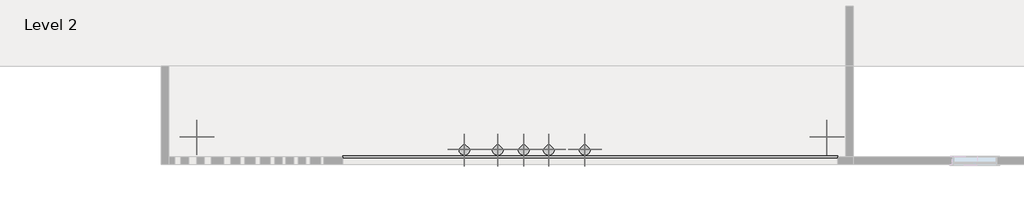
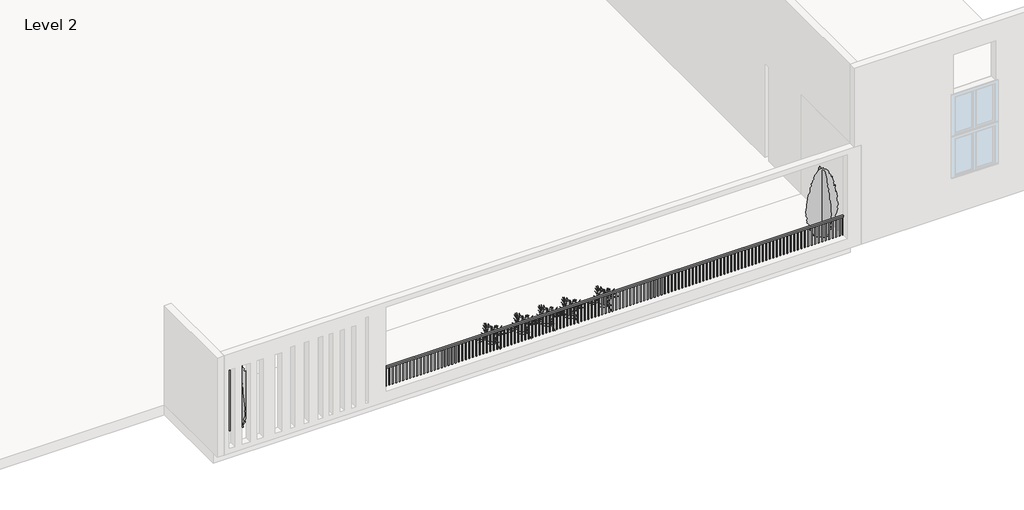
# One storey, part 2 of 2: 7 geographic elements, 1 railing.
"""IFC4 building model written with IfcOpenShell, lengths in millimetres."""

from ifc_helpers import new_model, si_unit, frame, origin, place, context, project, spatial, polyline, outline, extrude, transform, mapped, element, save
from components import rpc_plant_tropical_agave_1_5_93a2a214, rpc_tree_conifer_chinese_juniper_7_1b9786cd

model = new_model("IFC4")

# Units and contexts
model_context = context("Model", 3, world=origin())
ifc_project = project(units=[si_unit("LENGTHUNIT", "METRE", prefix="MILLI")], contexts=[model_context])

# Site, building, storey
site = spatial("IfcSite", under=ifc_project)
building = spatial("IfcBuilding", under=site)
storey = spatial("IfcBuildingStorey", under=building, Name="Level 2", Elevation=3200.4)

# Geographic elements
placement = place(None, origin())
rpc_plant_tropical_agave_1_5_shape = rpc_plant_tropical_agave_1_5_93a2a214(model_context)
element("IfcGeographicElement", 1, ObjectType="RPC Plant - Tropical : Agave - 1.5'", at=placement, inside=storey, context=model_context, shape_type="MappedRepresentation", body=[
    mapped(rpc_plant_tropical_agave_1_5_shape, transform((-1518.2073975, -18818.2462052, 3657.6), x_axis=(1.0, 0.0, 0.0), y_axis=(0.0, 1.0, 0.0), z_axis=(0.0, 0.0, 1.0))),
])
element("IfcGeographicElement", 2, ObjectType="RPC Plant - Tropical : Agave - 1.5'", at=placement, inside=storey, context=model_context, shape_type="MappedRepresentation", body=[
    mapped(rpc_plant_tropical_agave_1_5_shape, transform((-616.8826315, -18818.2462052, 3657.6), x_axis=(1.0, 0.0, 0.0), y_axis=(0.0, 1.0, 0.0), z_axis=(0.0, 0.0, 1.0))),
])
element("IfcGeographicElement", 3, ObjectType="RPC Plant - Tropical : Agave - 1.5'", at=placement, inside=storey, context=model_context, shape_type="MappedRepresentation", body=[
    mapped(rpc_plant_tropical_agave_1_5_shape, transform((88.759784, -18818.2462052, 3657.6), x_axis=(1.0, 0.0, 0.0), y_axis=(0.0, 1.0, 0.0), z_axis=(0.0, 0.0, 1.0))),
])
element("IfcGeographicElement", 4, ObjectType="RPC Plant - Tropical : Agave - 1.5'", at=placement, inside=storey, context=model_context, shape_type="MappedRepresentation", body=[
    mapped(rpc_plant_tropical_agave_1_5_shape, transform((764.7533585, -18818.2462052, 3657.6), x_axis=(1.0, 0.0, 0.0), y_axis=(0.0, 1.0, 0.0), z_axis=(0.0, 0.0, 1.0))),
])
element("IfcGeographicElement", 5, ObjectType="RPC Plant - Tropical : Agave - 1.5'", at=placement, inside=storey, context=model_context, shape_type="MappedRepresentation", body=[
    mapped(rpc_plant_tropical_agave_1_5_shape, transform((1745.1760973, -18818.2462052, 3657.6), x_axis=(1.0, 0.0, 0.0), y_axis=(0.0, 1.0, 0.0), z_axis=(0.0, 0.0, 1.0))),
])
rpc_tree_conifer_chinese_juniper_7_shape = rpc_tree_conifer_chinese_juniper_7_1b9786cd(model_context)
element("IfcGeographicElement", 6, ObjectType="RPC Tree - Conifer : Chinese Juniper - 7'", at=placement, inside=storey, context=model_context, shape_type="MappedRepresentation", body=[
    mapped(rpc_tree_conifer_chinese_juniper_7_shape, transform((8298.1794262, -18476.470124, 3200.4), x_axis=(1.0, 0.0, 0.0), y_axis=(0.0, 1.0, 0.0), z_axis=(0.0, 0.0, 1.0))),
])
element("IfcGeographicElement", 7, ObjectType="RPC Tree - Conifer : Chinese Juniper - 7'", at=placement, inside=storey, context=model_context, shape_type="MappedRepresentation", body=[
    mapped(rpc_tree_conifer_chinese_juniper_7_shape, transform((-8770.6205738, -18476.470124, 3200.4), x_axis=(1.0, 0.0, 0.0), y_axis=(0.0, 1.0, 0.0), z_axis=(0.0, 0.0, 1.0))),
])

# Railing
element("IfcRailing", 8, ObjectType="Handrail - Rectangular", at=placement, inside=storey, context=model_context, shape_type="SweptSolid", body=[
    extrude(outline(polyline([(-4809.1668389, -19046.8462052), (-4809.1668389, -18996.0462052), (8602.0331611, -18996.0462052), (8602.0331611, -19046.8462052), (-4809.1668389, -19046.8462052)])), frame((0.0, 0.0, 4064.0), z_axis=(0.0, 0.0, 1.0), x_axis=(1.0, 0.0, 0.0)), (0.0, 0.0, 1.0), 50.8),
    extrude(outline(polyline([(8490.9081611, -19030.9712052), (8490.9081611, -19011.9212052), (8509.9581611, -19011.9212052), (8509.9581611, -19030.9712052), (8490.9081611, -19030.9712052)])), frame((0.0, 0.0, 3200.4), z_axis=(0.0, 0.0, 1.0), x_axis=(1.0, 0.0, 0.0)), (0.0, 0.0, 1.0), 863.6),
    extrude(outline(polyline([(8389.3081611, -19030.9712052), (8389.3081611, -19011.9212052), (8408.3581611, -19011.9212052), (8408.3581611, -19030.9712052), (8389.3081611, -19030.9712052)])), frame((0.0, 0.0, 3200.4), z_axis=(0.0, 0.0, 1.0), x_axis=(1.0, 0.0, 0.0)), (0.0, 0.0, 1.0), 863.6),
    extrude(outline(polyline([(8287.7081611, -19030.9712052), (8287.7081611, -19011.9212052), (8306.7581611, -19011.9212052), (8306.7581611, -19030.9712052), (8287.7081611, -19030.9712052)])), frame((0.0, 0.0, 3200.4), z_axis=(0.0, 0.0, 1.0), x_axis=(1.0, 0.0, 0.0)), (0.0, 0.0, 1.0), 863.6),
    extrude(outline(polyline([(8186.1081611, -19030.9712052), (8186.1081611, -19011.9212052), (8205.1581611, -19011.9212052), (8205.1581611, -19030.9712052), (8186.1081611, -19030.9712052)])), frame((0.0, 0.0, 3200.4), z_axis=(0.0, 0.0, 1.0), x_axis=(1.0, 0.0, 0.0)), (0.0, 0.0, 1.0), 863.6),
    extrude(outline(polyline([(8084.5081611, -19030.9712052), (8084.5081611, -19011.9212052), (8103.5581611, -19011.9212052), (8103.5581611, -19030.9712052), (8084.5081611, -19030.9712052)])), frame((0.0, 0.0, 3200.4), z_axis=(0.0, 0.0, 1.0), x_axis=(1.0, 0.0, 0.0)), (0.0, 0.0, 1.0), 863.6),
    extrude(outline(polyline([(7982.9081611, -19030.9712052), (7982.9081611, -19011.9212052), (8001.9581611, -19011.9212052), (8001.9581611, -19030.9712052), (7982.9081611, -19030.9712052)])), frame((0.0, 0.0, 3200.4), z_axis=(0.0, 0.0, 1.0), x_axis=(1.0, 0.0, 0.0)), (0.0, 0.0, 1.0), 863.6),
    extrude(outline(polyline([(7881.3081611, -19030.9712052), (7881.3081611, -19011.9212052), (7900.3581611, -19011.9212052), (7900.3581611, -19030.9712052), (7881.3081611, -19030.9712052)])), frame((0.0, 0.0, 3200.4), z_axis=(0.0, 0.0, 1.0), x_axis=(1.0, 0.0, 0.0)), (0.0, 0.0, 1.0), 863.6),
    extrude(outline(polyline([(7779.7081611, -19030.9712052), (7779.7081611, -19011.9212052), (7798.7581611, -19011.9212052), (7798.7581611, -19030.9712052), (7779.7081611, -19030.9712052)])), frame((0.0, 0.0, 3200.4), z_axis=(0.0, 0.0, 1.0), x_axis=(1.0, 0.0, 0.0)), (0.0, 0.0, 1.0), 863.6),
    extrude(outline(polyline([(7678.1081611, -19030.9712052), (7678.1081611, -19011.9212052), (7697.1581611, -19011.9212052), (7697.1581611, -19030.9712052), (7678.1081611, -19030.9712052)])), frame((0.0, 0.0, 3200.4), z_axis=(0.0, 0.0, 1.0), x_axis=(1.0, 0.0, 0.0)), (0.0, 0.0, 1.0), 863.6),
    extrude(outline(polyline([(7576.5081611, -19030.9712052), (7576.5081611, -19011.9212052), (7595.5581611, -19011.9212052), (7595.5581611, -19030.9712052), (7576.5081611, -19030.9712052)])), frame((0.0, 0.0, 3200.4), z_axis=(0.0, 0.0, 1.0), x_axis=(1.0, 0.0, 0.0)), (0.0, 0.0, 1.0), 863.6),
    extrude(outline(polyline([(7474.9081611, -19030.9712052), (7474.9081611, -19011.9212052), (7493.9581611, -19011.9212052), (7493.9581611, -19030.9712052), (7474.9081611, -19030.9712052)])), frame((0.0, 0.0, 3200.4), z_axis=(0.0, 0.0, 1.0), x_axis=(1.0, 0.0, 0.0)), (0.0, 0.0, 1.0), 863.6),
    extrude(outline(polyline([(7373.3081611, -19030.9712052), (7373.3081611, -19011.9212052), (7392.3581611, -19011.9212052), (7392.3581611, -19030.9712052), (7373.3081611, -19030.9712052)])), frame((0.0, 0.0, 3200.4), z_axis=(0.0, 0.0, 1.0), x_axis=(1.0, 0.0, 0.0)), (0.0, 0.0, 1.0), 863.6),
    extrude(outline(polyline([(7271.7081611, -19030.9712052), (7271.7081611, -19011.9212052), (7290.7581611, -19011.9212052), (7290.7581611, -19030.9712052), (7271.7081611, -19030.9712052)])), frame((0.0, 0.0, 3200.4), z_axis=(0.0, 0.0, 1.0), x_axis=(1.0, 0.0, 0.0)), (0.0, 0.0, 1.0), 863.6),
    extrude(outline(polyline([(7170.1081611, -19030.9712052), (7170.1081611, -19011.9212052), (7189.1581611, -19011.9212052), (7189.1581611, -19030.9712052), (7170.1081611, -19030.9712052)])), frame((0.0, 0.0, 3200.4), z_axis=(0.0, 0.0, 1.0), x_axis=(1.0, 0.0, 0.0)), (0.0, 0.0, 1.0), 863.6),
    extrude(outline(polyline([(7068.5081611, -19030.9712052), (7068.5081611, -19011.9212052), (7087.5581611, -19011.9212052), (7087.5581611, -19030.9712052), (7068.5081611, -19030.9712052)])), frame((0.0, 0.0, 3200.4), z_axis=(0.0, 0.0, 1.0), x_axis=(1.0, 0.0, 0.0)), (0.0, 0.0, 1.0), 863.6),
    extrude(outline(polyline([(6966.9081611, -19030.9712052), (6966.9081611, -19011.9212052), (6985.9581611, -19011.9212052), (6985.9581611, -19030.9712052), (6966.9081611, -19030.9712052)])), frame((0.0, 0.0, 3200.4), z_axis=(0.0, 0.0, 1.0), x_axis=(1.0, 0.0, 0.0)), (0.0, 0.0, 1.0), 863.6),
    extrude(outline(polyline([(6865.3081611, -19030.9712052), (6865.3081611, -19011.9212052), (6884.3581611, -19011.9212052), (6884.3581611, -19030.9712052), (6865.3081611, -19030.9712052)])), frame((0.0, 0.0, 3200.4), z_axis=(0.0, 0.0, 1.0), x_axis=(1.0, 0.0, 0.0)), (0.0, 0.0, 1.0), 863.6),
    extrude(outline(polyline([(6763.7081611, -19030.9712052), (6763.7081611, -19011.9212052), (6782.7581611, -19011.9212052), (6782.7581611, -19030.9712052), (6763.7081611, -19030.9712052)])), frame((0.0, 0.0, 3200.4), z_axis=(0.0, 0.0, 1.0), x_axis=(1.0, 0.0, 0.0)), (0.0, 0.0, 1.0), 863.6),
    extrude(outline(polyline([(6662.1081611, -19030.9712052), (6662.1081611, -19011.9212052), (6681.1581611, -19011.9212052), (6681.1581611, -19030.9712052), (6662.1081611, -19030.9712052)])), frame((0.0, 0.0, 3200.4), z_axis=(0.0, 0.0, 1.0), x_axis=(1.0, 0.0, 0.0)), (0.0, 0.0, 1.0), 863.6),
    extrude(outline(polyline([(6560.5081611, -19030.9712052), (6560.5081611, -19011.9212052), (6579.5581611, -19011.9212052), (6579.5581611, -19030.9712052), (6560.5081611, -19030.9712052)])), frame((0.0, 0.0, 3200.4), z_axis=(0.0, 0.0, 1.0), x_axis=(1.0, 0.0, 0.0)), (0.0, 0.0, 1.0), 863.6),
    extrude(outline(polyline([(6458.9081611, -19030.9712052), (6458.9081611, -19011.9212052), (6477.9581611, -19011.9212052), (6477.9581611, -19030.9712052), (6458.9081611, -19030.9712052)])), frame((0.0, 0.0, 3200.4), z_axis=(0.0, 0.0, 1.0), x_axis=(1.0, 0.0, 0.0)), (0.0, 0.0, 1.0), 863.6),
    extrude(outline(polyline([(6357.3081611, -19030.9712052), (6357.3081611, -19011.9212052), (6376.3581611, -19011.9212052), (6376.3581611, -19030.9712052), (6357.3081611, -19030.9712052)])), frame((0.0, 0.0, 3200.4), z_axis=(0.0, 0.0, 1.0), x_axis=(1.0, 0.0, 0.0)), (0.0, 0.0, 1.0), 863.6),
    extrude(outline(polyline([(6255.7081611, -19030.9712052), (6255.7081611, -19011.9212052), (6274.7581611, -19011.9212052), (6274.7581611, -19030.9712052), (6255.7081611, -19030.9712052)])), frame((0.0, 0.0, 3200.4), z_axis=(0.0, 0.0, 1.0), x_axis=(1.0, 0.0, 0.0)), (0.0, 0.0, 1.0), 863.6),
    extrude(outline(polyline([(6154.1081611, -19030.9712052), (6154.1081611, -19011.9212052), (6173.1581611, -19011.9212052), (6173.1581611, -19030.9712052), (6154.1081611, -19030.9712052)])), frame((0.0, 0.0, 3200.4), z_axis=(0.0, 0.0, 1.0), x_axis=(1.0, 0.0, 0.0)), (0.0, 0.0, 1.0), 863.6),
    extrude(outline(polyline([(6052.5081611, -19030.9712052), (6052.5081611, -19011.9212052), (6071.5581611, -19011.9212052), (6071.5581611, -19030.9712052), (6052.5081611, -19030.9712052)])), frame((0.0, 0.0, 3200.4), z_axis=(0.0, 0.0, 1.0), x_axis=(1.0, 0.0, 0.0)), (0.0, 0.0, 1.0), 863.6),
    extrude(outline(polyline([(5950.9081611, -19030.9712052), (5950.9081611, -19011.9212052), (5969.9581611, -19011.9212052), (5969.9581611, -19030.9712052), (5950.9081611, -19030.9712052)])), frame((0.0, 0.0, 3200.4), z_axis=(0.0, 0.0, 1.0), x_axis=(1.0, 0.0, 0.0)), (0.0, 0.0, 1.0), 863.6),
    extrude(outline(polyline([(5849.3081611, -19030.9712052), (5849.3081611, -19011.9212052), (5868.3581611, -19011.9212052), (5868.3581611, -19030.9712052), (5849.3081611, -19030.9712052)])), frame((0.0, 0.0, 3200.4), z_axis=(0.0, 0.0, 1.0), x_axis=(1.0, 0.0, 0.0)), (0.0, 0.0, 1.0), 863.6),
    extrude(outline(polyline([(5747.7081611, -19030.9712052), (5747.7081611, -19011.9212052), (5766.7581611, -19011.9212052), (5766.7581611, -19030.9712052), (5747.7081611, -19030.9712052)])), frame((0.0, 0.0, 3200.4), z_axis=(0.0, 0.0, 1.0), x_axis=(1.0, 0.0, 0.0)), (0.0, 0.0, 1.0), 863.6),
    extrude(outline(polyline([(5646.1081611, -19030.9712052), (5646.1081611, -19011.9212052), (5665.1581611, -19011.9212052), (5665.1581611, -19030.9712052), (5646.1081611, -19030.9712052)])), frame((0.0, 0.0, 3200.4), z_axis=(0.0, 0.0, 1.0), x_axis=(1.0, 0.0, 0.0)), (0.0, 0.0, 1.0), 863.6),
    extrude(outline(polyline([(5544.5081611, -19030.9712052), (5544.5081611, -19011.9212052), (5563.5581611, -19011.9212052), (5563.5581611, -19030.9712052), (5544.5081611, -19030.9712052)])), frame((0.0, 0.0, 3200.4), z_axis=(0.0, 0.0, 1.0), x_axis=(1.0, 0.0, 0.0)), (0.0, 0.0, 1.0), 863.6),
    extrude(outline(polyline([(5442.9081611, -19030.9712052), (5442.9081611, -19011.9212052), (5461.9581611, -19011.9212052), (5461.9581611, -19030.9712052), (5442.9081611, -19030.9712052)])), frame((0.0, 0.0, 3200.4), z_axis=(0.0, 0.0, 1.0), x_axis=(1.0, 0.0, 0.0)), (0.0, 0.0, 1.0), 863.6),
    extrude(outline(polyline([(5341.3081611, -19030.9712052), (5341.3081611, -19011.9212052), (5360.3581611, -19011.9212052), (5360.3581611, -19030.9712052), (5341.3081611, -19030.9712052)])), frame((0.0, 0.0, 3200.4), z_axis=(0.0, 0.0, 1.0), x_axis=(1.0, 0.0, 0.0)), (0.0, 0.0, 1.0), 863.6),
    extrude(outline(polyline([(5239.7081611, -19030.9712052), (5239.7081611, -19011.9212052), (5258.7581611, -19011.9212052), (5258.7581611, -19030.9712052), (5239.7081611, -19030.9712052)])), frame((0.0, 0.0, 3200.4), z_axis=(0.0, 0.0, 1.0), x_axis=(1.0, 0.0, 0.0)), (0.0, 0.0, 1.0), 863.6),
    extrude(outline(polyline([(5138.1081611, -19030.9712052), (5138.1081611, -19011.9212052), (5157.1581611, -19011.9212052), (5157.1581611, -19030.9712052), (5138.1081611, -19030.9712052)])), frame((0.0, 0.0, 3200.4), z_axis=(0.0, 0.0, 1.0), x_axis=(1.0, 0.0, 0.0)), (0.0, 0.0, 1.0), 863.6),
    extrude(outline(polyline([(5036.5081611, -19030.9712052), (5036.5081611, -19011.9212052), (5055.5581611, -19011.9212052), (5055.5581611, -19030.9712052), (5036.5081611, -19030.9712052)])), frame((0.0, 0.0, 3200.4), z_axis=(0.0, 0.0, 1.0), x_axis=(1.0, 0.0, 0.0)), (0.0, 0.0, 1.0), 863.6),
    extrude(outline(polyline([(4934.9081611, -19030.9712052), (4934.9081611, -19011.9212052), (4953.9581611, -19011.9212052), (4953.9581611, -19030.9712052), (4934.9081611, -19030.9712052)])), frame((0.0, 0.0, 3200.4), z_axis=(0.0, 0.0, 1.0), x_axis=(1.0, 0.0, 0.0)), (0.0, 0.0, 1.0), 863.6),
    extrude(outline(polyline([(4833.3081611, -19030.9712052), (4833.3081611, -19011.9212052), (4852.3581611, -19011.9212052), (4852.3581611, -19030.9712052), (4833.3081611, -19030.9712052)])), frame((0.0, 0.0, 3200.4), z_axis=(0.0, 0.0, 1.0), x_axis=(1.0, 0.0, 0.0)), (0.0, 0.0, 1.0), 863.6),
    extrude(outline(polyline([(4731.7081611, -19030.9712052), (4731.7081611, -19011.9212052), (4750.7581611, -19011.9212052), (4750.7581611, -19030.9712052), (4731.7081611, -19030.9712052)])), frame((0.0, 0.0, 3200.4), z_axis=(0.0, 0.0, 1.0), x_axis=(1.0, 0.0, 0.0)), (0.0, 0.0, 1.0), 863.6),
    extrude(outline(polyline([(4630.1081611, -19030.9712052), (4630.1081611, -19011.9212052), (4649.1581611, -19011.9212052), (4649.1581611, -19030.9712052), (4630.1081611, -19030.9712052)])), frame((0.0, 0.0, 3200.4), z_axis=(0.0, 0.0, 1.0), x_axis=(1.0, 0.0, 0.0)), (0.0, 0.0, 1.0), 863.6),
    extrude(outline(polyline([(4528.5081611, -19030.9712052), (4528.5081611, -19011.9212052), (4547.5581611, -19011.9212052), (4547.5581611, -19030.9712052), (4528.5081611, -19030.9712052)])), frame((0.0, 0.0, 3200.4), z_axis=(0.0, 0.0, 1.0), x_axis=(1.0, 0.0, 0.0)), (0.0, 0.0, 1.0), 863.6),
    extrude(outline(polyline([(4426.9081611, -19030.9712052), (4426.9081611, -19011.9212052), (4445.9581611, -19011.9212052), (4445.9581611, -19030.9712052), (4426.9081611, -19030.9712052)])), frame((0.0, 0.0, 3200.4), z_axis=(0.0, 0.0, 1.0), x_axis=(1.0, 0.0, 0.0)), (0.0, 0.0, 1.0), 863.6),
    extrude(outline(polyline([(4325.3081611, -19030.9712052), (4325.3081611, -19011.9212052), (4344.3581611, -19011.9212052), (4344.3581611, -19030.9712052), (4325.3081611, -19030.9712052)])), frame((0.0, 0.0, 3200.4), z_axis=(0.0, 0.0, 1.0), x_axis=(1.0, 0.0, 0.0)), (0.0, 0.0, 1.0), 863.6),
    extrude(outline(polyline([(4223.7081611, -19030.9712052), (4223.7081611, -19011.9212052), (4242.7581611, -19011.9212052), (4242.7581611, -19030.9712052), (4223.7081611, -19030.9712052)])), frame((0.0, 0.0, 3200.4), z_axis=(0.0, 0.0, 1.0), x_axis=(1.0, 0.0, 0.0)), (0.0, 0.0, 1.0), 863.6),
    extrude(outline(polyline([(4122.1081611, -19030.9712052), (4122.1081611, -19011.9212052), (4141.1581611, -19011.9212052), (4141.1581611, -19030.9712052), (4122.1081611, -19030.9712052)])), frame((0.0, 0.0, 3200.4), z_axis=(0.0, 0.0, 1.0), x_axis=(1.0, 0.0, 0.0)), (0.0, 0.0, 1.0), 863.6),
    extrude(outline(polyline([(4020.5081611, -19030.9712052), (4020.5081611, -19011.9212052), (4039.5581611, -19011.9212052), (4039.5581611, -19030.9712052), (4020.5081611, -19030.9712052)])), frame((0.0, 0.0, 3200.4), z_axis=(0.0, 0.0, 1.0), x_axis=(1.0, 0.0, 0.0)), (0.0, 0.0, 1.0), 863.6),
    extrude(outline(polyline([(3918.9081611, -19030.9712052), (3918.9081611, -19011.9212052), (3937.9581611, -19011.9212052), (3937.9581611, -19030.9712052), (3918.9081611, -19030.9712052)])), frame((0.0, 0.0, 3200.4), z_axis=(0.0, 0.0, 1.0), x_axis=(1.0, 0.0, 0.0)), (0.0, 0.0, 1.0), 863.6),
    extrude(outline(polyline([(3817.3081611, -19030.9712052), (3817.3081611, -19011.9212052), (3836.3581611, -19011.9212052), (3836.3581611, -19030.9712052), (3817.3081611, -19030.9712052)])), frame((0.0, 0.0, 3200.4), z_axis=(0.0, 0.0, 1.0), x_axis=(1.0, 0.0, 0.0)), (0.0, 0.0, 1.0), 863.6),
    extrude(outline(polyline([(3715.7081611, -19030.9712052), (3715.7081611, -19011.9212052), (3734.7581611, -19011.9212052), (3734.7581611, -19030.9712052), (3715.7081611, -19030.9712052)])), frame((0.0, 0.0, 3200.4), z_axis=(0.0, 0.0, 1.0), x_axis=(1.0, 0.0, 0.0)), (0.0, 0.0, 1.0), 863.6),
    extrude(outline(polyline([(3614.1081611, -19030.9712052), (3614.1081611, -19011.9212052), (3633.1581611, -19011.9212052), (3633.1581611, -19030.9712052), (3614.1081611, -19030.9712052)])), frame((0.0, 0.0, 3200.4), z_axis=(0.0, 0.0, 1.0), x_axis=(1.0, 0.0, 0.0)), (0.0, 0.0, 1.0), 863.6),
    extrude(outline(polyline([(3512.5081611, -19030.9712052), (3512.5081611, -19011.9212052), (3531.5581611, -19011.9212052), (3531.5581611, -19030.9712052), (3512.5081611, -19030.9712052)])), frame((0.0, 0.0, 3200.4), z_axis=(0.0, 0.0, 1.0), x_axis=(1.0, 0.0, 0.0)), (0.0, 0.0, 1.0), 863.6),
    extrude(outline(polyline([(3410.9081611, -19030.9712052), (3410.9081611, -19011.9212052), (3429.9581611, -19011.9212052), (3429.9581611, -19030.9712052), (3410.9081611, -19030.9712052)])), frame((0.0, 0.0, 3200.4), z_axis=(0.0, 0.0, 1.0), x_axis=(1.0, 0.0, 0.0)), (0.0, 0.0, 1.0), 863.6),
    extrude(outline(polyline([(3309.3081611, -19030.9712052), (3309.3081611, -19011.9212052), (3328.3581611, -19011.9212052), (3328.3581611, -19030.9712052), (3309.3081611, -19030.9712052)])), frame((0.0, 0.0, 3200.4), z_axis=(0.0, 0.0, 1.0), x_axis=(1.0, 0.0, 0.0)), (0.0, 0.0, 1.0), 863.6),
    extrude(outline(polyline([(3207.7081611, -19030.9712052), (3207.7081611, -19011.9212052), (3226.7581611, -19011.9212052), (3226.7581611, -19030.9712052), (3207.7081611, -19030.9712052)])), frame((0.0, 0.0, 3200.4), z_axis=(0.0, 0.0, 1.0), x_axis=(1.0, 0.0, 0.0)), (0.0, 0.0, 1.0), 863.6),
    extrude(outline(polyline([(3106.1081611, -19030.9712052), (3106.1081611, -19011.9212052), (3125.1581611, -19011.9212052), (3125.1581611, -19030.9712052), (3106.1081611, -19030.9712052)])), frame((0.0, 0.0, 3200.4), z_axis=(0.0, 0.0, 1.0), x_axis=(1.0, 0.0, 0.0)), (0.0, 0.0, 1.0), 863.6),
    extrude(outline(polyline([(3004.5081611, -19030.9712052), (3004.5081611, -19011.9212052), (3023.5581611, -19011.9212052), (3023.5581611, -19030.9712052), (3004.5081611, -19030.9712052)])), frame((0.0, 0.0, 3200.4), z_axis=(0.0, 0.0, 1.0), x_axis=(1.0, 0.0, 0.0)), (0.0, 0.0, 1.0), 863.6),
    extrude(outline(polyline([(2902.9081611, -19030.9712052), (2902.9081611, -19011.9212052), (2921.9581611, -19011.9212052), (2921.9581611, -19030.9712052), (2902.9081611, -19030.9712052)])), frame((0.0, 0.0, 3200.4), z_axis=(0.0, 0.0, 1.0), x_axis=(1.0, 0.0, 0.0)), (0.0, 0.0, 1.0), 863.6),
    extrude(outline(polyline([(2801.3081611, -19030.9712052), (2801.3081611, -19011.9212052), (2820.3581611, -19011.9212052), (2820.3581611, -19030.9712052), (2801.3081611, -19030.9712052)])), frame((0.0, 0.0, 3200.4), z_axis=(0.0, 0.0, 1.0), x_axis=(1.0, 0.0, 0.0)), (0.0, 0.0, 1.0), 863.6),
    extrude(outline(polyline([(2699.7081611, -19030.9712052), (2699.7081611, -19011.9212052), (2718.7581611, -19011.9212052), (2718.7581611, -19030.9712052), (2699.7081611, -19030.9712052)])), frame((0.0, 0.0, 3200.4), z_axis=(0.0, 0.0, 1.0), x_axis=(1.0, 0.0, 0.0)), (0.0, 0.0, 1.0), 863.6),
    extrude(outline(polyline([(2598.1081611, -19030.9712052), (2598.1081611, -19011.9212052), (2617.1581611, -19011.9212052), (2617.1581611, -19030.9712052), (2598.1081611, -19030.9712052)])), frame((0.0, 0.0, 3200.4), z_axis=(0.0, 0.0, 1.0), x_axis=(1.0, 0.0, 0.0)), (0.0, 0.0, 1.0), 863.6),
    extrude(outline(polyline([(2496.5081611, -19030.9712052), (2496.5081611, -19011.9212052), (2515.5581611, -19011.9212052), (2515.5581611, -19030.9712052), (2496.5081611, -19030.9712052)])), frame((0.0, 0.0, 3200.4), z_axis=(0.0, 0.0, 1.0), x_axis=(1.0, 0.0, 0.0)), (0.0, 0.0, 1.0), 863.6),
    extrude(outline(polyline([(2394.9081611, -19030.9712052), (2394.9081611, -19011.9212052), (2413.9581611, -19011.9212052), (2413.9581611, -19030.9712052), (2394.9081611, -19030.9712052)])), frame((0.0, 0.0, 3200.4), z_axis=(0.0, 0.0, 1.0), x_axis=(1.0, 0.0, 0.0)), (0.0, 0.0, 1.0), 863.6),
    extrude(outline(polyline([(2293.3081611, -19030.9712052), (2293.3081611, -19011.9212052), (2312.3581611, -19011.9212052), (2312.3581611, -19030.9712052), (2293.3081611, -19030.9712052)])), frame((0.0, 0.0, 3200.4), z_axis=(0.0, 0.0, 1.0), x_axis=(1.0, 0.0, 0.0)), (0.0, 0.0, 1.0), 863.6),
    extrude(outline(polyline([(2191.7081611, -19030.9712052), (2191.7081611, -19011.9212052), (2210.7581611, -19011.9212052), (2210.7581611, -19030.9712052), (2191.7081611, -19030.9712052)])), frame((0.0, 0.0, 3200.4), z_axis=(0.0, 0.0, 1.0), x_axis=(1.0, 0.0, 0.0)), (0.0, 0.0, 1.0), 863.6),
    extrude(outline(polyline([(2090.1081611, -19030.9712052), (2090.1081611, -19011.9212052), (2109.1581611, -19011.9212052), (2109.1581611, -19030.9712052), (2090.1081611, -19030.9712052)])), frame((0.0, 0.0, 3200.4), z_axis=(0.0, 0.0, 1.0), x_axis=(1.0, 0.0, 0.0)), (0.0, 0.0, 1.0), 863.6),
    extrude(outline(polyline([(1988.5081611, -19030.9712052), (1988.5081611, -19011.9212052), (2007.5581611, -19011.9212052), (2007.5581611, -19030.9712052), (1988.5081611, -19030.9712052)])), frame((0.0, 0.0, 3200.4), z_axis=(0.0, 0.0, 1.0), x_axis=(1.0, 0.0, 0.0)), (0.0, 0.0, 1.0), 863.6),
    extrude(outline(polyline([(1886.9081611, -19030.9712052), (1886.9081611, -19011.9212052), (1905.9581611, -19011.9212052), (1905.9581611, -19030.9712052), (1886.9081611, -19030.9712052)])), frame((0.0, 0.0, 3200.4), z_axis=(0.0, 0.0, 1.0), x_axis=(1.0, 0.0, 0.0)), (0.0, 0.0, 1.0), 863.6),
    extrude(outline(polyline([(1785.3081611, -19030.9712052), (1785.3081611, -19011.9212052), (1804.3581611, -19011.9212052), (1804.3581611, -19030.9712052), (1785.3081611, -19030.9712052)])), frame((0.0, 0.0, 3200.4), z_axis=(0.0, 0.0, 1.0), x_axis=(1.0, 0.0, 0.0)), (0.0, 0.0, 1.0), 863.6),
    extrude(outline(polyline([(1683.7081611, -19030.9712052), (1683.7081611, -19011.9212052), (1702.7581611, -19011.9212052), (1702.7581611, -19030.9712052), (1683.7081611, -19030.9712052)])), frame((0.0, 0.0, 3200.4), z_axis=(0.0, 0.0, 1.0), x_axis=(1.0, 0.0, 0.0)), (0.0, 0.0, 1.0), 863.6),
    extrude(outline(polyline([(1582.1081611, -19030.9712052), (1582.1081611, -19011.9212052), (1601.1581611, -19011.9212052), (1601.1581611, -19030.9712052), (1582.1081611, -19030.9712052)])), frame((0.0, 0.0, 3200.4), z_axis=(0.0, 0.0, 1.0), x_axis=(1.0, 0.0, 0.0)), (0.0, 0.0, 1.0), 863.6),
    extrude(outline(polyline([(1480.5081611, -19030.9712052), (1480.5081611, -19011.9212052), (1499.5581611, -19011.9212052), (1499.5581611, -19030.9712052), (1480.5081611, -19030.9712052)])), frame((0.0, 0.0, 3200.4), z_axis=(0.0, 0.0, 1.0), x_axis=(1.0, 0.0, 0.0)), (0.0, 0.0, 1.0), 863.6),
    extrude(outline(polyline([(1378.9081611, -19030.9712052), (1378.9081611, -19011.9212052), (1397.9581611, -19011.9212052), (1397.9581611, -19030.9712052), (1378.9081611, -19030.9712052)])), frame((0.0, 0.0, 3200.4), z_axis=(0.0, 0.0, 1.0), x_axis=(1.0, 0.0, 0.0)), (0.0, 0.0, 1.0), 863.6),
    extrude(outline(polyline([(1277.3081611, -19030.9712052), (1277.3081611, -19011.9212052), (1296.3581611, -19011.9212052), (1296.3581611, -19030.9712052), (1277.3081611, -19030.9712052)])), frame((0.0, 0.0, 3200.4), z_axis=(0.0, 0.0, 1.0), x_axis=(1.0, 0.0, 0.0)), (0.0, 0.0, 1.0), 863.6),
    extrude(outline(polyline([(1175.7081611, -19030.9712052), (1175.7081611, -19011.9212052), (1194.7581611, -19011.9212052), (1194.7581611, -19030.9712052), (1175.7081611, -19030.9712052)])), frame((0.0, 0.0, 3200.4), z_axis=(0.0, 0.0, 1.0), x_axis=(1.0, 0.0, 0.0)), (0.0, 0.0, 1.0), 863.6),
    extrude(outline(polyline([(1074.1081611, -19030.9712052), (1074.1081611, -19011.9212052), (1093.1581611, -19011.9212052), (1093.1581611, -19030.9712052), (1074.1081611, -19030.9712052)])), frame((0.0, 0.0, 3200.4), z_axis=(0.0, 0.0, 1.0), x_axis=(1.0, 0.0, 0.0)), (0.0, 0.0, 1.0), 863.6),
    extrude(outline(polyline([(972.5081611, -19030.9712052), (972.5081611, -19011.9212052), (991.5581611, -19011.9212052), (991.5581611, -19030.9712052), (972.5081611, -19030.9712052)])), frame((0.0, 0.0, 3200.4), z_axis=(0.0, 0.0, 1.0), x_axis=(1.0, 0.0, 0.0)), (0.0, 0.0, 1.0), 863.6),
    extrude(outline(polyline([(870.9081611, -19030.9712052), (870.9081611, -19011.9212052), (889.9581611, -19011.9212052), (889.9581611, -19030.9712052), (870.9081611, -19030.9712052)])), frame((0.0, 0.0, 3200.4), z_axis=(0.0, 0.0, 1.0), x_axis=(1.0, 0.0, 0.0)), (0.0, 0.0, 1.0), 863.6),
    extrude(outline(polyline([(769.3081611, -19030.9712052), (769.3081611, -19011.9212052), (788.3581611, -19011.9212052), (788.3581611, -19030.9712052), (769.3081611, -19030.9712052)])), frame((0.0, 0.0, 3200.4), z_axis=(0.0, 0.0, 1.0), x_axis=(1.0, 0.0, 0.0)), (0.0, 0.0, 1.0), 863.6),
    extrude(outline(polyline([(667.7081611, -19030.9712052), (667.7081611, -19011.9212052), (686.7581611, -19011.9212052), (686.7581611, -19030.9712052), (667.7081611, -19030.9712052)])), frame((0.0, 0.0, 3200.4), z_axis=(0.0, 0.0, 1.0), x_axis=(1.0, 0.0, 0.0)), (0.0, 0.0, 1.0), 863.6),
    extrude(outline(polyline([(566.1081611, -19030.9712052), (566.1081611, -19011.9212052), (585.1581611, -19011.9212052), (585.1581611, -19030.9712052), (566.1081611, -19030.9712052)])), frame((0.0, 0.0, 3200.4), z_axis=(0.0, 0.0, 1.0), x_axis=(1.0, 0.0, 0.0)), (0.0, 0.0, 1.0), 863.6),
    extrude(outline(polyline([(464.5081611, -19030.9712052), (464.5081611, -19011.9212052), (483.5581611, -19011.9212052), (483.5581611, -19030.9712052), (464.5081611, -19030.9712052)])), frame((0.0, 0.0, 3200.4), z_axis=(0.0, 0.0, 1.0), x_axis=(1.0, 0.0, 0.0)), (0.0, 0.0, 1.0), 863.6),
    extrude(outline(polyline([(362.9081611, -19030.9712052), (362.9081611, -19011.9212052), (381.9581611, -19011.9212052), (381.9581611, -19030.9712052), (362.9081611, -19030.9712052)])), frame((0.0, 0.0, 3200.4), z_axis=(0.0, 0.0, 1.0), x_axis=(1.0, 0.0, 0.0)), (0.0, 0.0, 1.0), 863.6),
    extrude(outline(polyline([(261.3081611, -19030.9712052), (261.3081611, -19011.9212052), (280.3581611, -19011.9212052), (280.3581611, -19030.9712052), (261.3081611, -19030.9712052)])), frame((0.0, 0.0, 3200.4), z_axis=(0.0, 0.0, 1.0), x_axis=(1.0, 0.0, 0.0)), (0.0, 0.0, 1.0), 863.6),
    extrude(outline(polyline([(159.7081611, -19030.9712052), (159.7081611, -19011.9212052), (178.7581611, -19011.9212052), (178.7581611, -19030.9712052), (159.7081611, -19030.9712052)])), frame((0.0, 0.0, 3200.4), z_axis=(0.0, 0.0, 1.0), x_axis=(1.0, 0.0, 0.0)), (0.0, 0.0, 1.0), 863.6),
    extrude(outline(polyline([(58.1081611, -19030.9712052), (58.1081611, -19011.9212052), (77.1581611, -19011.9212052), (77.1581611, -19030.9712052), (58.1081611, -19030.9712052)])), frame((0.0, 0.0, 3200.4), z_axis=(0.0, 0.0, 1.0), x_axis=(1.0, 0.0, 0.0)), (0.0, 0.0, 1.0), 863.6),
    extrude(outline(polyline([(-43.4918389, -19030.9712052), (-43.4918389, -19011.9212052), (-24.4418389, -19011.9212052), (-24.4418389, -19030.9712052), (-43.4918389, -19030.9712052)])), frame((0.0, 0.0, 3200.4), z_axis=(0.0, 0.0, 1.0), x_axis=(1.0, 0.0, 0.0)), (0.0, 0.0, 1.0), 863.6),
    extrude(outline(polyline([(-145.0918389, -19030.9712052), (-145.0918389, -19011.9212052), (-126.0418389, -19011.9212052), (-126.0418389, -19030.9712052), (-145.0918389, -19030.9712052)])), frame((0.0, 0.0, 3200.4), z_axis=(0.0, 0.0, 1.0), x_axis=(1.0, 0.0, 0.0)), (0.0, 0.0, 1.0), 863.6),
    extrude(outline(polyline([(-246.6918389, -19030.9712052), (-246.6918389, -19011.9212052), (-227.6418389, -19011.9212052), (-227.6418389, -19030.9712052), (-246.6918389, -19030.9712052)])), frame((0.0, 0.0, 3200.4), z_axis=(0.0, 0.0, 1.0), x_axis=(1.0, 0.0, 0.0)), (0.0, 0.0, 1.0), 863.6),
    extrude(outline(polyline([(-348.2918389, -19030.9712052), (-348.2918389, -19011.9212052), (-329.2418389, -19011.9212052), (-329.2418389, -19030.9712052), (-348.2918389, -19030.9712052)])), frame((0.0, 0.0, 3200.4), z_axis=(0.0, 0.0, 1.0), x_axis=(1.0, 0.0, 0.0)), (0.0, 0.0, 1.0), 863.6),
    extrude(outline(polyline([(-449.8918389, -19030.9712052), (-449.8918389, -19011.9212052), (-430.8418389, -19011.9212052), (-430.8418389, -19030.9712052), (-449.8918389, -19030.9712052)])), frame((0.0, 0.0, 3200.4), z_axis=(0.0, 0.0, 1.0), x_axis=(1.0, 0.0, 0.0)), (0.0, 0.0, 1.0), 863.6),
    extrude(outline(polyline([(-551.4918389, -19030.9712052), (-551.4918389, -19011.9212052), (-532.4418389, -19011.9212052), (-532.4418389, -19030.9712052), (-551.4918389, -19030.9712052)])), frame((0.0, 0.0, 3200.4), z_axis=(0.0, 0.0, 1.0), x_axis=(1.0, 0.0, 0.0)), (0.0, 0.0, 1.0), 863.6),
    extrude(outline(polyline([(-653.0918389, -19030.9712052), (-653.0918389, -19011.9212052), (-634.0418389, -19011.9212052), (-634.0418389, -19030.9712052), (-653.0918389, -19030.9712052)])), frame((0.0, 0.0, 3200.4), z_axis=(0.0, 0.0, 1.0), x_axis=(1.0, 0.0, 0.0)), (0.0, 0.0, 1.0), 863.6),
    extrude(outline(polyline([(-754.6918389, -19030.9712052), (-754.6918389, -19011.9212052), (-735.6418389, -19011.9212052), (-735.6418389, -19030.9712052), (-754.6918389, -19030.9712052)])), frame((0.0, 0.0, 3200.4), z_axis=(0.0, 0.0, 1.0), x_axis=(1.0, 0.0, 0.0)), (0.0, 0.0, 1.0), 863.6),
    extrude(outline(polyline([(-856.2918389, -19030.9712052), (-856.2918389, -19011.9212052), (-837.2418389, -19011.9212052), (-837.2418389, -19030.9712052), (-856.2918389, -19030.9712052)])), frame((0.0, 0.0, 3200.4), z_axis=(0.0, 0.0, 1.0), x_axis=(1.0, 0.0, 0.0)), (0.0, 0.0, 1.0), 863.6),
    extrude(outline(polyline([(-957.8918389, -19030.9712052), (-957.8918389, -19011.9212052), (-938.8418389, -19011.9212052), (-938.8418389, -19030.9712052), (-957.8918389, -19030.9712052)])), frame((0.0, 0.0, 3200.4), z_axis=(0.0, 0.0, 1.0), x_axis=(1.0, 0.0, 0.0)), (0.0, 0.0, 1.0), 863.6),
    extrude(outline(polyline([(-1059.4918389, -19030.9712052), (-1059.4918389, -19011.9212052), (-1040.4418389, -19011.9212052), (-1040.4418389, -19030.9712052), (-1059.4918389, -19030.9712052)])), frame((0.0, 0.0, 3200.4), z_axis=(0.0, 0.0, 1.0), x_axis=(1.0, 0.0, 0.0)), (0.0, 0.0, 1.0), 863.6),
    extrude(outline(polyline([(-1161.0918389, -19030.9712052), (-1161.0918389, -19011.9212052), (-1142.0418389, -19011.9212052), (-1142.0418389, -19030.9712052), (-1161.0918389, -19030.9712052)])), frame((0.0, 0.0, 3200.4), z_axis=(0.0, 0.0, 1.0), x_axis=(1.0, 0.0, 0.0)), (0.0, 0.0, 1.0), 863.6),
    extrude(outline(polyline([(-1262.6918389, -19030.9712052), (-1262.6918389, -19011.9212052), (-1243.6418389, -19011.9212052), (-1243.6418389, -19030.9712052), (-1262.6918389, -19030.9712052)])), frame((0.0, 0.0, 3200.4), z_axis=(0.0, 0.0, 1.0), x_axis=(1.0, 0.0, 0.0)), (0.0, 0.0, 1.0), 863.6),
    extrude(outline(polyline([(-1364.2918389, -19030.9712052), (-1364.2918389, -19011.9212052), (-1345.2418389, -19011.9212052), (-1345.2418389, -19030.9712052), (-1364.2918389, -19030.9712052)])), frame((0.0, 0.0, 3200.4), z_axis=(0.0, 0.0, 1.0), x_axis=(1.0, 0.0, 0.0)), (0.0, 0.0, 1.0), 863.6),
    extrude(outline(polyline([(-1465.8918389, -19030.9712052), (-1465.8918389, -19011.9212052), (-1446.8418389, -19011.9212052), (-1446.8418389, -19030.9712052), (-1465.8918389, -19030.9712052)])), frame((0.0, 0.0, 3200.4), z_axis=(0.0, 0.0, 1.0), x_axis=(1.0, 0.0, 0.0)), (0.0, 0.0, 1.0), 863.6),
    extrude(outline(polyline([(-1567.4918389, -19030.9712052), (-1567.4918389, -19011.9212052), (-1548.4418389, -19011.9212052), (-1548.4418389, -19030.9712052), (-1567.4918389, -19030.9712052)])), frame((0.0, 0.0, 3200.4), z_axis=(0.0, 0.0, 1.0), x_axis=(1.0, 0.0, 0.0)), (0.0, 0.0, 1.0), 863.6),
    extrude(outline(polyline([(-1669.0918389, -19030.9712052), (-1669.0918389, -19011.9212052), (-1650.0418389, -19011.9212052), (-1650.0418389, -19030.9712052), (-1669.0918389, -19030.9712052)])), frame((0.0, 0.0, 3200.4), z_axis=(0.0, 0.0, 1.0), x_axis=(1.0, 0.0, 0.0)), (0.0, 0.0, 1.0), 863.6),
    extrude(outline(polyline([(-1770.6918389, -19030.9712052), (-1770.6918389, -19011.9212052), (-1751.6418389, -19011.9212052), (-1751.6418389, -19030.9712052), (-1770.6918389, -19030.9712052)])), frame((0.0, 0.0, 3200.4), z_axis=(0.0, 0.0, 1.0), x_axis=(1.0, 0.0, 0.0)), (0.0, 0.0, 1.0), 863.6),
    extrude(outline(polyline([(-1872.2918389, -19030.9712052), (-1872.2918389, -19011.9212052), (-1853.2418389, -19011.9212052), (-1853.2418389, -19030.9712052), (-1872.2918389, -19030.9712052)])), frame((0.0, 0.0, 3200.4), z_axis=(0.0, 0.0, 1.0), x_axis=(1.0, 0.0, 0.0)), (0.0, 0.0, 1.0), 863.6),
    extrude(outline(polyline([(-1973.8918389, -19030.9712052), (-1973.8918389, -19011.9212052), (-1954.8418389, -19011.9212052), (-1954.8418389, -19030.9712052), (-1973.8918389, -19030.9712052)])), frame((0.0, 0.0, 3200.4), z_axis=(0.0, 0.0, 1.0), x_axis=(1.0, 0.0, 0.0)), (0.0, 0.0, 1.0), 863.6),
    extrude(outline(polyline([(-2075.4918389, -19030.9712052), (-2075.4918389, -19011.9212052), (-2056.4418389, -19011.9212052), (-2056.4418389, -19030.9712052), (-2075.4918389, -19030.9712052)])), frame((0.0, 0.0, 3200.4), z_axis=(0.0, 0.0, 1.0), x_axis=(1.0, 0.0, 0.0)), (0.0, 0.0, 1.0), 863.6),
    extrude(outline(polyline([(-2177.0918389, -19030.9712052), (-2177.0918389, -19011.9212052), (-2158.0418389, -19011.9212052), (-2158.0418389, -19030.9712052), (-2177.0918389, -19030.9712052)])), frame((0.0, 0.0, 3200.4), z_axis=(0.0, 0.0, 1.0), x_axis=(1.0, 0.0, 0.0)), (0.0, 0.0, 1.0), 863.6),
    extrude(outline(polyline([(-2278.6918389, -19030.9712052), (-2278.6918389, -19011.9212052), (-2259.6418389, -19011.9212052), (-2259.6418389, -19030.9712052), (-2278.6918389, -19030.9712052)])), frame((0.0, 0.0, 3200.4), z_axis=(0.0, 0.0, 1.0), x_axis=(1.0, 0.0, 0.0)), (0.0, 0.0, 1.0), 863.6),
    extrude(outline(polyline([(-2380.2918389, -19030.9712052), (-2380.2918389, -19011.9212052), (-2361.2418389, -19011.9212052), (-2361.2418389, -19030.9712052), (-2380.2918389, -19030.9712052)])), frame((0.0, 0.0, 3200.4), z_axis=(0.0, 0.0, 1.0), x_axis=(1.0, 0.0, 0.0)), (0.0, 0.0, 1.0), 863.6),
    extrude(outline(polyline([(-2481.8918389, -19030.9712052), (-2481.8918389, -19011.9212052), (-2462.8418389, -19011.9212052), (-2462.8418389, -19030.9712052), (-2481.8918389, -19030.9712052)])), frame((0.0, 0.0, 3200.4), z_axis=(0.0, 0.0, 1.0), x_axis=(1.0, 0.0, 0.0)), (0.0, 0.0, 1.0), 863.6),
    extrude(outline(polyline([(-2583.4918389, -19030.9712052), (-2583.4918389, -19011.9212052), (-2564.4418389, -19011.9212052), (-2564.4418389, -19030.9712052), (-2583.4918389, -19030.9712052)])), frame((0.0, 0.0, 3200.4), z_axis=(0.0, 0.0, 1.0), x_axis=(1.0, 0.0, 0.0)), (0.0, 0.0, 1.0), 863.6),
    extrude(outline(polyline([(-2685.0918389, -19030.9712052), (-2685.0918389, -19011.9212052), (-2666.0418389, -19011.9212052), (-2666.0418389, -19030.9712052), (-2685.0918389, -19030.9712052)])), frame((0.0, 0.0, 3200.4), z_axis=(0.0, 0.0, 1.0), x_axis=(1.0, 0.0, 0.0)), (0.0, 0.0, 1.0), 863.6),
    extrude(outline(polyline([(-2786.6918389, -19030.9712052), (-2786.6918389, -19011.9212052), (-2767.6418389, -19011.9212052), (-2767.6418389, -19030.9712052), (-2786.6918389, -19030.9712052)])), frame((0.0, 0.0, 3200.4), z_axis=(0.0, 0.0, 1.0), x_axis=(1.0, 0.0, 0.0)), (0.0, 0.0, 1.0), 863.6),
    extrude(outline(polyline([(-2888.2918389, -19030.9712052), (-2888.2918389, -19011.9212052), (-2869.2418389, -19011.9212052), (-2869.2418389, -19030.9712052), (-2888.2918389, -19030.9712052)])), frame((0.0, 0.0, 3200.4), z_axis=(0.0, 0.0, 1.0), x_axis=(1.0, 0.0, 0.0)), (0.0, 0.0, 1.0), 863.6),
    extrude(outline(polyline([(-2989.8918389, -19030.9712052), (-2989.8918389, -19011.9212052), (-2970.8418389, -19011.9212052), (-2970.8418389, -19030.9712052), (-2989.8918389, -19030.9712052)])), frame((0.0, 0.0, 3200.4), z_axis=(0.0, 0.0, 1.0), x_axis=(1.0, 0.0, 0.0)), (0.0, 0.0, 1.0), 863.6),
    extrude(outline(polyline([(-3091.4918389, -19030.9712052), (-3091.4918389, -19011.9212052), (-3072.4418389, -19011.9212052), (-3072.4418389, -19030.9712052), (-3091.4918389, -19030.9712052)])), frame((0.0, 0.0, 3200.4), z_axis=(0.0, 0.0, 1.0), x_axis=(1.0, 0.0, 0.0)), (0.0, 0.0, 1.0), 863.6),
    extrude(outline(polyline([(-3193.0918389, -19030.9712052), (-3193.0918389, -19011.9212052), (-3174.0418389, -19011.9212052), (-3174.0418389, -19030.9712052), (-3193.0918389, -19030.9712052)])), frame((0.0, 0.0, 3200.4), z_axis=(0.0, 0.0, 1.0), x_axis=(1.0, 0.0, 0.0)), (0.0, 0.0, 1.0), 863.6),
    extrude(outline(polyline([(-3294.6918389, -19030.9712052), (-3294.6918389, -19011.9212052), (-3275.6418389, -19011.9212052), (-3275.6418389, -19030.9712052), (-3294.6918389, -19030.9712052)])), frame((0.0, 0.0, 3200.4), z_axis=(0.0, 0.0, 1.0), x_axis=(1.0, 0.0, 0.0)), (0.0, 0.0, 1.0), 863.6),
    extrude(outline(polyline([(-3396.2918389, -19030.9712052), (-3396.2918389, -19011.9212052), (-3377.2418389, -19011.9212052), (-3377.2418389, -19030.9712052), (-3396.2918389, -19030.9712052)])), frame((0.0, 0.0, 3200.4), z_axis=(0.0, 0.0, 1.0), x_axis=(1.0, 0.0, 0.0)), (0.0, 0.0, 1.0), 863.6),
    extrude(outline(polyline([(-3497.8918389, -19030.9712052), (-3497.8918389, -19011.9212052), (-3478.8418389, -19011.9212052), (-3478.8418389, -19030.9712052), (-3497.8918389, -19030.9712052)])), frame((0.0, 0.0, 3200.4), z_axis=(0.0, 0.0, 1.0), x_axis=(1.0, 0.0, 0.0)), (0.0, 0.0, 1.0), 863.6),
    extrude(outline(polyline([(-3599.4918389, -19030.9712052), (-3599.4918389, -19011.9212052), (-3580.4418389, -19011.9212052), (-3580.4418389, -19030.9712052), (-3599.4918389, -19030.9712052)])), frame((0.0, 0.0, 3200.4), z_axis=(0.0, 0.0, 1.0), x_axis=(1.0, 0.0, 0.0)), (0.0, 0.0, 1.0), 863.6),
    extrude(outline(polyline([(-3701.0918389, -19030.9712052), (-3701.0918389, -19011.9212052), (-3682.0418389, -19011.9212052), (-3682.0418389, -19030.9712052), (-3701.0918389, -19030.9712052)])), frame((0.0, 0.0, 3200.4), z_axis=(0.0, 0.0, 1.0), x_axis=(1.0, 0.0, 0.0)), (0.0, 0.0, 1.0), 863.6),
    extrude(outline(polyline([(-3802.6918389, -19030.9712052), (-3802.6918389, -19011.9212052), (-3783.6418389, -19011.9212052), (-3783.6418389, -19030.9712052), (-3802.6918389, -19030.9712052)])), frame((0.0, 0.0, 3200.4), z_axis=(0.0, 0.0, 1.0), x_axis=(1.0, 0.0, 0.0)), (0.0, 0.0, 1.0), 863.6),
    extrude(outline(polyline([(-3904.2918389, -19030.9712052), (-3904.2918389, -19011.9212052), (-3885.2418389, -19011.9212052), (-3885.2418389, -19030.9712052), (-3904.2918389, -19030.9712052)])), frame((0.0, 0.0, 3200.4), z_axis=(0.0, 0.0, 1.0), x_axis=(1.0, 0.0, 0.0)), (0.0, 0.0, 1.0), 863.6),
    extrude(outline(polyline([(-4005.8918389, -19030.9712052), (-4005.8918389, -19011.9212052), (-3986.8418389, -19011.9212052), (-3986.8418389, -19030.9712052), (-4005.8918389, -19030.9712052)])), frame((0.0, 0.0, 3200.4), z_axis=(0.0, 0.0, 1.0), x_axis=(1.0, 0.0, 0.0)), (0.0, 0.0, 1.0), 863.6),
    extrude(outline(polyline([(-4107.4918389, -19030.9712052), (-4107.4918389, -19011.9212052), (-4088.4418389, -19011.9212052), (-4088.4418389, -19030.9712052), (-4107.4918389, -19030.9712052)])), frame((0.0, 0.0, 3200.4), z_axis=(0.0, 0.0, 1.0), x_axis=(1.0, 0.0, 0.0)), (0.0, 0.0, 1.0), 863.6),
    extrude(outline(polyline([(-4209.0918389, -19030.9712052), (-4209.0918389, -19011.9212052), (-4190.0418389, -19011.9212052), (-4190.0418389, -19030.9712052), (-4209.0918389, -19030.9712052)])), frame((0.0, 0.0, 3200.4), z_axis=(0.0, 0.0, 1.0), x_axis=(1.0, 0.0, 0.0)), (0.0, 0.0, 1.0), 863.6),
    extrude(outline(polyline([(-4310.6918389, -19030.9712052), (-4310.6918389, -19011.9212052), (-4291.6418389, -19011.9212052), (-4291.6418389, -19030.9712052), (-4310.6918389, -19030.9712052)])), frame((0.0, 0.0, 3200.4), z_axis=(0.0, 0.0, 1.0), x_axis=(1.0, 0.0, 0.0)), (0.0, 0.0, 1.0), 863.6),
    extrude(outline(polyline([(-4412.2918389, -19030.9712052), (-4412.2918389, -19011.9212052), (-4393.2418389, -19011.9212052), (-4393.2418389, -19030.9712052), (-4412.2918389, -19030.9712052)])), frame((0.0, 0.0, 3200.4), z_axis=(0.0, 0.0, 1.0), x_axis=(1.0, 0.0, 0.0)), (0.0, 0.0, 1.0), 863.6),
    extrude(outline(polyline([(-4513.8918389, -19030.9712052), (-4513.8918389, -19011.9212052), (-4494.8418389, -19011.9212052), (-4494.8418389, -19030.9712052), (-4513.8918389, -19030.9712052)])), frame((0.0, 0.0, 3200.4), z_axis=(0.0, 0.0, 1.0), x_axis=(1.0, 0.0, 0.0)), (0.0, 0.0, 1.0), 863.6),
    extrude(outline(polyline([(-4615.4918389, -19030.9712052), (-4615.4918389, -19011.9212052), (-4596.4418389, -19011.9212052), (-4596.4418389, -19030.9712052), (-4615.4918389, -19030.9712052)])), frame((0.0, 0.0, 3200.4), z_axis=(0.0, 0.0, 1.0), x_axis=(1.0, 0.0, 0.0)), (0.0, 0.0, 1.0), 863.6),
    extrude(outline(polyline([(-4717.0918389, -19030.9712052), (-4717.0918389, -19011.9212052), (-4698.0418389, -19011.9212052), (-4698.0418389, -19030.9712052), (-4717.0918389, -19030.9712052)])), frame((0.0, 0.0, 3200.4), z_axis=(0.0, 0.0, 1.0), x_axis=(1.0, 0.0, 0.0)), (0.0, 0.0, 1.0), 863.6),
    extrude(outline(polyline([(8582.9831611, -19030.9712052), (8582.9831611, -19011.9212052), (8602.0331611, -19011.9212052), (8602.0331611, -19030.9712052), (8582.9831611, -19030.9712052)])), frame((0.0, 0.0, 3200.4), z_axis=(0.0, 0.0, 1.0), x_axis=(1.0, 0.0, 0.0)), (0.0, 0.0, 1.0), 863.6),
    extrude(outline(polyline([(-4809.1668389, -19030.9712052), (-4809.1668389, -19011.9212052), (-4790.1168389, -19011.9212052), (-4790.1168389, -19030.9712052), (-4809.1668389, -19030.9712052)])), frame((0.0, 0.0, 3200.4), z_axis=(0.0, 0.0, 1.0), x_axis=(1.0, 0.0, 0.0)), (0.0, 0.0, 1.0), 863.6),
])

save(model, "model.ifc")

# Revit data of these elements
# Type "RPC Plant - Tropical : Agave - 1.5'"
#   built-in parameter 1005198 = "{2, 15},{39, RPC-16-G1GJ-63FX-7K5P-N000-ST1L-LVER-AU},{1, 0},{1, 0},{2, 13},{1, 8},{5, Color},{1, 0},{1, 0},{3, 0.8},{3, 0.8},{3, 0.8},{1, 8},{7, BBoxMin},{1, 0},{1, 0},{1, 0},{1, 0},{1, 0},{1, 8},{7, BBoxMax},{1, 0},{1, 0},{1, 0},{1, 0},{1, 0},{2, 11},{9, RPCTypeId},{1, 0},{1, 0},{39, RPC-16-G1GJ-63FX-7K5P-N000-ST1L-LVER-AU},{1, 6},{14, RPCPlantHeight},{1, 0},{1, 0},{3, 1.5},{2, 11},{7, keyword},{1, 0},{1, 0},{35, :RPCs:Plants [General]:Geometry:RPC},{2, 11},{8, category},{1, 0},{1, 0},{16, Plants [General]},{2, 11},{12, LocalizedUID},{1, 0},{1, 0},{5, Agave},{2, 14},{6, Height},{1, 0},{1, 0},{3, 1.5},{1, 2},{16, Cast Reflections},{1, 0},{1, 0},{1, 0},{1, 2},{12, Cast Shadows},{1, 0},{1, 0},{1, 1},{1, 2},{9, Lock View},{1, 0},{1, 0},{1, 0},{1, 4},{5, ViewC},{1, 0},{1, 0},{1, 0},{21, assetlibrary_base.fbx},{1, 5},"
#   built-in parameter 1005195 = "RPC-16-G1GJ-63FX-7K5P-N000-ST1L-LVER-AU"
#   Type Comments = "Agave"
#   Assembly Code = "G2050500"
#   Height = 1' - 6"
#   Default Elevation = 0
# Type "RPC Tree - Conifer : Chinese Juniper - 7'"
#   built-in parameter 1005198 = "{2, 15},{39, RPC-16-FUM3-UUQ0-UBF0-N000-ST1L-LVER-AU},{1, 0},{1, 0},{2, 13},{1, 8},{5, Color},{1, 0},{1, 0},{3, 0.8},{3, 0.8},{3, 0.8},{1, 8},{7, BBoxMin},{1, 0},{1, 0},{1, 0},{1, 0},{1, 0},{1, 8},{7, BBoxMax},{1, 0},{1, 0},{1, 0},{1, 0},{1, 0},{2, 11},{9, RPCTypeId},{1, 0},{1, 0},{39, RPC-16-FUM3-UUQ0-UBF0-N000-ST1L-LVER-AU},{1, 6},{14, RPCPlantHeight},{1, 0},{1, 0},{1, 7},{2, 11},{7, keyword},{1, 0},{1, 0},{34, :RPCs:Trees [General]:Geometry:RPC},{2, 11},{8, category},{1, 0},{1, 0},{15, Trees [General]},{2, 11},{12, LocalizedUID},{1, 0},{1, 0},{15, Chinese Juniper},{2, 14},{6, Height},{1, 0},{1, 0},{1, 7},{1, 2},{16, Cast Reflections},{1, 0},{1, 0},{1, 0},{1, 2},{12, Cast Shadows},{1, 0},{1, 0},{1, 1},{1, 2},{9, Lock View},{1, 0},{1, 0},{1, 0},{1, 4},{5, ViewC},{1, 0},{1, 0},{1, 0},{21, assetlibrary_base.fbx},{1, 5},"
#   built-in parameter 1005195 = "RPC-16-FUM3-UUQ0-UBF0-N000-ST1L-LVER-AU"
#   Type Comments = "Chinese Juniper"
#   Assembly Code = "G2050500"
#   Height = 7' - 0"
#   Description = (empty or 0)
#   Default Elevation = 0
# Type "Handrail - Rectangular"
#   Assembly Code = "C2010400"
#   built-in parameter 1008612 = 0.0416667 (stored number, unit not read)
#   built-in parameter 1008611 = 0.0416667 (stored number, unit not read)
#   built-in parameter 1008609 = 0.333333 (stored number, unit not read)
#   built-in parameter 1008604 = 0.166667 (stored number, unit not read)
#   built-in parameter 1008603 = 0.166667 (stored number, unit not read)
#   Railing Height = 3' - 0"
#   built-in parameter 1008630 = 2
#   built-in parameter 1008610 = 2
#   built-in parameter 1008618 = Baluster - Square : 3/4"
# Elements 1, 2, 3, 4, 5 (IfcGeographicElement, "RPC Plant - Tropical : Agave - 1.5'")
#   Phase Created = New Construction
# Elements 6, 7 (IfcGeographicElement, "RPC Tree - Conifer : Chinese Juniper - 7'")
#   Phase Created = New Construction
# Element 8 (IfcRailing, "Handrail - Rectangular")
#   Phase Created = New Construction
